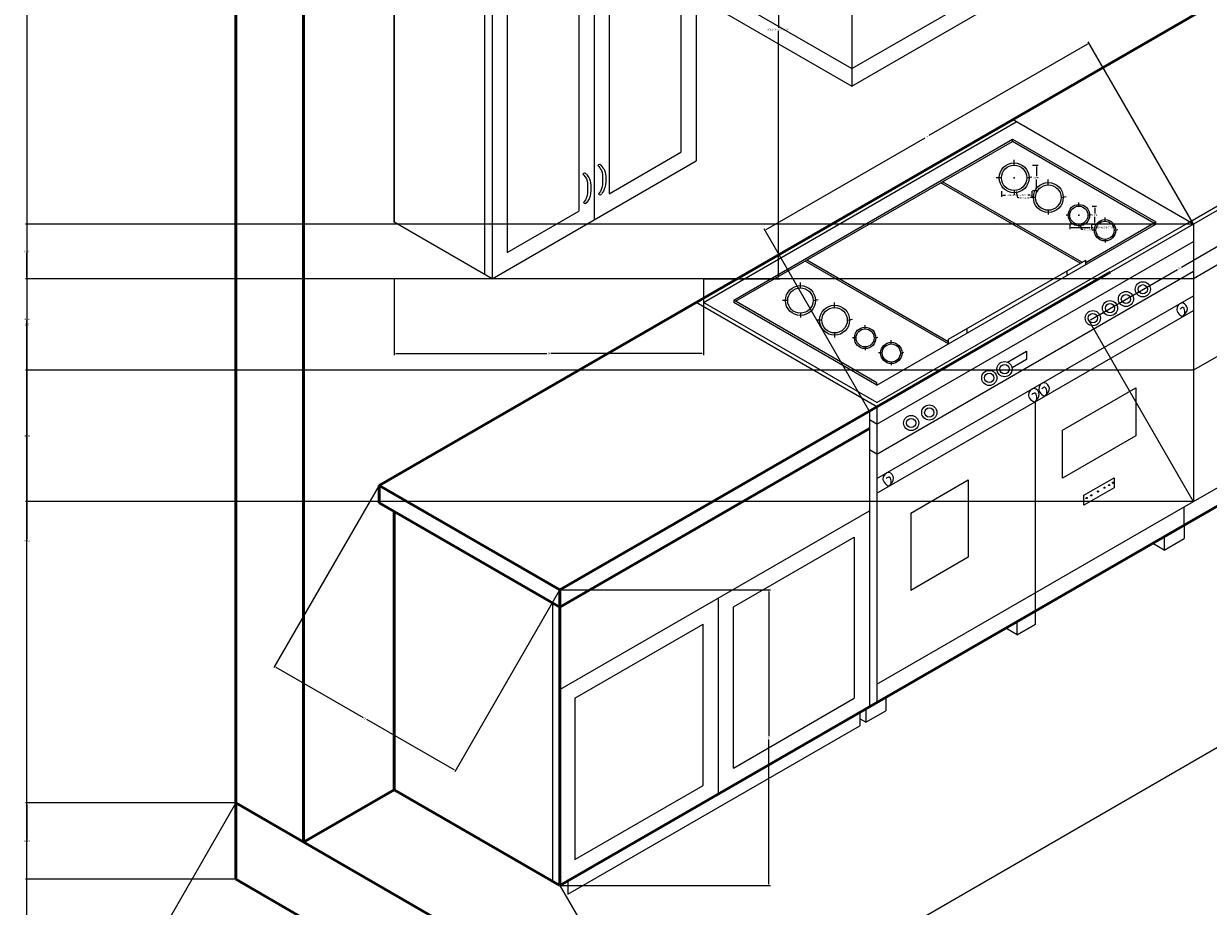
# Model space of a CAD drawing. Units: inches. Extents: x 4150 to 4636, y 2169 to 2592.
# Tile 2 of 8: x 4150 to 4286, y 2337 to 2438. Entities that reach past the tile are written whole.
import ezdxf

# ---------------------------------------------------------------- set-up
doc = ezdxf.new("R2010")
doc.units = ezdxf.units.IN
for name, color, linetype, lineweight in [('A-ANNO-DIMS', 2, 'Continuous', 18), ('A-EQPM', 6, 'Continuous', 25), ('A-FLOR-CASE', 3, 'Continuous', 25), ('A-FLOR-FIXT', 8, 'Continuous', 18), ('A-WALL', 7, 'Continuous', 50)]:
    doc.layers.add(name, color=color, linetype=linetype, lineweight=lineweight)
doc.styles.get("Standard").update_dxf_attribs({"font": 'arial.ttf'})
doc.dimstyles.get("Standard").update_dxf_attribs({"dimtxt": 0.18, "dimasz": 0.18, "dimexe": 0.18, "dimexo": 0.0625, "dimgap": 0.09, "dimtad": 0, "dimtih": 1, "dimtoh": 1, "dimdec": 4, "dimzin": 0, "dimdsep": 46, "dimtxsty": 'Standard', "dimcen": 0.09, "dimadec": 0, "dimazin": 0, "dimtfac": 1, "dimtdec": 4, "dimtofl": 0, "dimtmove": 0, "dimatfit": 3, "dimfxl": 1, "dimtolj": 1, "dimtzin": 0, "dimarcsym": 0})

# ---------------------------------------------------------------- blocks, each defined once
blk = doc.blocks.new('CUBOARD 2')
for p, q in [((4217.63, 2465.79), (4218.5, 2466.29)), ((4217.63, 2463.68), (4217.63, 2465.79)), ((4226.29, 2460.79), (4217.63, 2465.79)), ((4228.02, 2460.79), (4218.5, 2466.29)), ((4195.16, 2450.71), (4217.63, 2463.68)), ((4224.46, 2459.74), (4217.63, 2463.68)), ((4201.99, 2446.77), (4226.29, 2460.79)), ((4202.86, 2446.27), (4228.02, 2460.79)), ((4202.86, 2446.27), (4228.02, 2460.79)), ((4228.02, 2460.79), (4228.02, 2457.68)), ((4202.86, 2443.15), (4228.02, 2457.68)), ((4227.16, 2457.18), (4227.16, 2422.52)), ((4217.17, 2449.42), (4225.43, 2454.18)), ((4225.43, 2454.18), (4225.43, 2423.52)), ((4192.47, 2452.27), (4202.86, 2446.27)), ((4192.47, 2449.15), (4192.47, 2452.27)), ((4215.44, 2450.42), (4215.44, 2415.75)), ((4192.47, 2449.15), (4202.86, 2443.15)), ((4192.47, 2449.15), (4192.47, 2415.49)), ((4217.17, 2449.42), (4217.17, 2418.75)), ((4205.46, 2442.65), (4213.71, 2447.42)), ((4213.71, 2447.42), (4213.71, 2416.75)), ((4202.86, 2446.27), (4202.86, 2443.15)), ((4202.86, 2443.15), (4202.86, 2446.27)), ((4203.72, 2443.65), (4203.72, 2408.99)), ((4202.86, 2443.15), (4202.86, 2409.49)), ((4205.46, 2442.65), (4205.46, 2411.99)), ((4217.17, 2418.75), (4225.43, 2423.52)), ((4203.72, 2408.99), (4227.16, 2422.52)), ((4205.46, 2411.99), (4213.71, 2416.75)), ((4203.72, 2408.99), (4192.47, 2415.49))]:
    blk.add_line(p, q)
for centre, radius, start, end in [((4216.06, 2421.92), 0.201, 29.3135, 156.7087), ((4214.34, 2420.93), 0.201, 29.3135, 156.7087), ((4214.42, 2417.84), 0.198, 207.8897, 338.1325), ((4216.13, 2418.83), 0.198, 207.8897, 338.1325)]:
    blk.add_arc(centre, radius, start, end)
for points in [[(4215.87, 2422), (4216.03, 2421.82), (4216.41, 2421.39), (4216.43, 2420.34), (4216.42, 2419.36), (4216.06, 2418.86), (4215.96, 2418.73)], [(4216.23, 2422.02), (4216.39, 2421.84), (4216.77, 2421.41), (4216.79, 2420.36), (4216.78, 2419.38), (4216.41, 2418.88), (4216.32, 2418.75)], [(4214.16, 2421.01), (4214.31, 2420.83), (4214.69, 2420.4), (4214.71, 2419.35), (4214.71, 2418.37), (4214.34, 2417.87), (4214.24, 2417.74)], [(4214.52, 2421.03), (4214.67, 2420.85), (4215.05, 2420.42), (4215.07, 2419.37), (4215.07, 2418.38), (4214.7, 2417.89), (4214.6, 2417.76)]]:
    blk.add_open_spline(points, degree=3, knots=[0, 0, 0, 0, 0.695815, 1.679053, 3.025679, 3.502598, 3.502598, 3.502598, 3.502598])
blk = doc.blocks.new('AIR FRESH')
for p, q in [((4253.73, 2486.84), (4245.07, 2491.84)), ((4236.41, 2486.84), (4236.41, 2462.84)), ((4245.07, 2481.84), (4236.41, 2486.84)), ((4245.07, 2481.84), (4253.73, 2486.84)), ((4253.73, 2486.84), (4253.73, 2462.84)), ((4245.07, 2457.84), (4245.07, 2481.84)), ((4238.41, 2480.59), (4238.41, 2478.46)), ((4238.41, 2480.59), (4242.22, 2478.39)), ((4238.41, 2478.46), (4242.22, 2476.26)), ((4242.22, 2476.26), (4242.22, 2478.39)), ((4236.41, 2462.84), (4228.02, 2457.99)), ((4236.41, 2462.84), (4245.07, 2457.84)), ((4253.73, 2462.84), (4245.07, 2457.84)), ((4253.73, 2462.84), (4275.13, 2450.48)), ((4245.07, 2457.84), (4245.07, 2433.13)), ((4245.07, 2433.13), (4275.13, 2450.48)), ((4275.13, 2450.48), (4275.13, 2448.48)), ((4245.07, 2431.13), (4275.13, 2448.48)), ((4227.16, 2443.47), (4245.07, 2433.13)), ((4227.16, 2441.47), (4245.07, 2431.13)), ((4245.07, 2433.13), (4245.07, 2431.13))]:
    blk.add_line(p, q)
for centre in [(4239.24, 2478.91), (4240.29, 2478.31), (4241.32, 2477.71)]:
    blk.add_circle(centre, 0.313)
blk = doc.blocks.new('KNOB-A')
blk.add_line((2.93, 1.46), (3.5, 1.57))
blk.add_circle((1.46, 1.46), 1.46)
blk = doc.blocks.new('KNOB-B')
blk.add_line((2.09, 1.04), (2.5, 1.12))
blk.add_circle((1.04, 1.04), 1.04)
blk = doc.blocks.new('*D26')
at = {"layer": 'A-ANNO-DIMS', "color": 0, "lineweight": -2, "transparency": 16777216}
for p, q in [((4262.25, 2419.06), (4262.25, 2418.41)), ((4265.75, 2419.06), (4265.75, 2418.41)), ((4262.43, 2418.59), (4262.73, 2418.59)), ((4265.57, 2418.59), (4265.27, 2418.59))]:
    blk.add_line(p, q, dxfattribs=at)
at = {"layer": 'A-ANNO-DIMS', "color": 0, "transparency": 16777216}
for points in [[(4262.43, 2418.62), (4262.43, 2418.56), (4262.25, 2418.59)], [(4265.57, 2418.62), (4265.57, 2418.56), (4265.75, 2418.59)]]:
    blk.add_solid(points, dxfattribs=at)
at = {"layer": 'Defpoints', "color": 0, "transparency": 16777216}
for p in [(4262.25, 2419.12), (4265.75, 2419.12), (4265.75, 2418.59)]:
    blk.add_point(p, dxfattribs=at)
at = {"layer": 'A-ANNO-DIMS', "color": 0, "transparency": 16777216, "insert": (4264, 2418.59), "char_height": 0.18, "attachment_point": 5}
blk.add_mtext('\\A1;HOB KNOB A 4 TYP.', dxfattribs=at)
blk = doc.blocks.new('*D27')
at = {"layer": 'A-ANNO-DIMS', "color": 0, "lineweight": -2, "transparency": 16777216}
for p, q in [((4265.81, 2422.05), (4266.46, 2422.05)), ((4266.28, 2421.87), (4266.28, 2420.77)), ((4266.28, 2419.3), (4266.28, 2420.4)), ((4265.81, 2419.12), (4266.46, 2419.12))]:
    blk.add_line(p, q, dxfattribs=at)
at = {"layer": 'A-ANNO-DIMS', "color": 0, "transparency": 16777216}
for points in [[(4266.25, 2421.87), (4266.31, 2421.87), (4266.28, 2422.05)], [(4266.25, 2419.3), (4266.31, 2419.3), (4266.28, 2419.12)]]:
    blk.add_solid(points, dxfattribs=at)
at = {"layer": 'Defpoints', "color": 0, "transparency": 16777216}
for p in [(4265.75, 2422.05), (4266.28, 2422.05), (4265.75, 2419.12)]:
    blk.add_point(p, dxfattribs=at)
at = {"layer": 'A-ANNO-DIMS', "color": 0, "transparency": 16777216, "insert": (4266.28, 2420.58), "char_height": 0.18, "attachment_point": 5}
blk.add_mtext('\\A1;3 TYP.', dxfattribs=at)
blk = doc.blocks.new('*D28')
at = {"layer": 'A-ANNO-DIMS', "color": 0, "lineweight": -2, "transparency": 16777216}
for p, q in [((4270.1, 2415.18), (4270.1, 2414.69)), ((4270.28, 2414.87), (4272.42, 2414.87)), ((4272.6, 2415.18), (4272.6, 2414.69)), ((4272.6, 2414.87), (4272.78, 2414.87))]:
    blk.add_line(p, q, dxfattribs=at)
at = {"layer": 'A-ANNO-DIMS', "color": 0, "transparency": 16777216}
for points in [[(4270.28, 2414.9), (4270.28, 2414.84), (4270.1, 2414.87)], [(4272.42, 2414.9), (4272.42, 2414.84), (4272.6, 2414.87)]]:
    blk.add_solid(points, dxfattribs=at)
at = {"layer": 'Defpoints', "color": 0, "transparency": 16777216}
for p in [(4270.1, 2415.25), (4272.6, 2415.25), (4272.6, 2414.87)]:
    blk.add_point(p, dxfattribs=at)
at = {"layer": 'A-ANNO-DIMS', "color": 0, "transparency": 16777216, "insert": (4274.05, 2414.87), "char_height": 0.18, "attachment_point": 5}
blk.add_mtext('\\A1;HOB KNOB B 2 TYP.', dxfattribs=at)
blk = doc.blocks.new('*D29')
at = {"layer": 'A-ANNO-DIMS', "color": 0, "lineweight": -2, "transparency": 16777216}
for p, q in [((4272.67, 2417.33), (4273.16, 2417.33)), ((4272.98, 2417.15), (4272.98, 2416.47)), ((4272.98, 2415.43), (4272.98, 2416.11)), ((4272.67, 2415.25), (4273.16, 2415.25))]:
    blk.add_line(p, q, dxfattribs=at)
at = {"layer": 'A-ANNO-DIMS', "color": 0, "transparency": 16777216}
for points in [[(4272.95, 2417.15), (4273.01, 2417.15), (4272.98, 2417.33)], [(4272.95, 2415.43), (4273.01, 2415.43), (4272.98, 2415.25)]]:
    blk.add_solid(points, dxfattribs=at)
at = {"layer": 'Defpoints', "color": 0, "transparency": 16777216}
for p in [(4272.6, 2417.33), (4272.98, 2417.33), (4272.6, 2415.25)]:
    blk.add_point(p, dxfattribs=at)
at = {"layer": 'A-ANNO-DIMS', "color": 0, "transparency": 16777216, "insert": (4272.98, 2416.29), "char_height": 0.18, "attachment_point": 5}
blk.add_mtext('\\A1;2 TYP.', dxfattribs=at)
blk = doc.blocks.new('*D34')
at = {"layer": 'A-ANNO-DIMS', "color": 0, "lineweight": -2, "transparency": 16777216}
for p, q in [((4228.09, 2466.29), (4236.8, 2466.29)), ((4236.62, 2466.11), (4236.62, 2437.82)), ((4236.62, 2409.17), (4236.62, 2437.46)), ((4228.09, 2408.99), (4236.8, 2408.99))]:
    blk.add_line(p, q, dxfattribs=at)
at = {"layer": 'A-ANNO-DIMS', "color": 0, "transparency": 16777216}
for points in [[(4236.59, 2466.11), (4236.65, 2466.11), (4236.62, 2466.29)], [(4236.59, 2409.17), (4236.65, 2409.17), (4236.62, 2408.99)]]:
    blk.add_solid(points, dxfattribs=at)
at = {"layer": 'Defpoints', "color": 0, "transparency": 16777216}
for p in [(4228.02, 2466.29), (4236.62, 2466.29), (4228.02, 2408.99)]:
    blk.add_point(p, dxfattribs=at)
at = {"layer": 'A-ANNO-DIMS', "color": 0, "transparency": 16777216, "insert": (4236.62, 2437.64), "char_height": 0.18, "attachment_point": 5}
blk.add_mtext('\\A1;WALL CUPBOARD 2 57', dxfattribs=at)
blk = doc.blocks.new('*D35')
at = {"layer": 'A-ANNO-DIMS', "color": 0, "lineweight": -2, "transparency": 16777216}
for p, q in [((4192.47, 2408.92), (4192.47, 2400.21)), ((4228.02, 2408.92), (4228.02, 2400.21)), ((4192.65, 2400.39), (4210.03, 2400.39)), ((4227.84, 2400.39), (4210.46, 2400.39))]:
    blk.add_line(p, q, dxfattribs=at)
at = {"layer": 'A-ANNO-DIMS', "color": 0, "transparency": 16777216}
for points in [[(4192.65, 2400.42), (4192.65, 2400.36), (4192.47, 2400.39)], [(4227.84, 2400.42), (4227.84, 2400.36), (4228.02, 2400.39)]]:
    blk.add_solid(points, dxfattribs=at)
at = {"layer": 'Defpoints', "color": 0, "transparency": 16777216}
for p in [(4192.47, 2408.99), (4228.02, 2408.99), (4228.02, 2400.39)]:
    blk.add_point(p, dxfattribs=at)
at = {"layer": 'A-ANNO-DIMS', "color": 0, "transparency": 16777216, "insert": (4210.25, 2400.39), "char_height": 0.18, "attachment_point": 5}
blk.add_mtext('\\A1;36', dxfattribs=at)
blk = doc.blocks.new('*D36')
at = {"layer": 'A-ANNO-DIMS', "color": 0, "lineweight": -2, "transparency": 16777216}
for p, q in [((4174.28, 2460.03), (4174.28, 2592.15)), ((4174.46, 2591.97), (4402.51, 2591.97)), ((4631.36, 2591.97), (4403.31, 2591.97)), ((4631.54, 2412.03), (4631.54, 2592.15))]:
    blk.add_line(p, q, dxfattribs=at)
at = {"layer": 'A-ANNO-DIMS', "color": 0, "transparency": 16777216}
for points in [[(4174.46, 2592), (4174.46, 2591.94), (4174.28, 2591.97)], [(4631.36, 2592), (4631.36, 2591.94), (4631.54, 2591.97)]]:
    blk.add_solid(points, dxfattribs=at)
at = {"layer": 'Defpoints', "color": 0, "transparency": 16777216}
for p in [(4631.54, 2591.97), (4174.28, 2459.97), (4631.54, 2411.97)]:
    blk.add_point(p, dxfattribs=at)
at = {"layer": 'A-ANNO-DIMS', "color": 0, "transparency": 16777216, "insert": (4402.91, 2591.97), "char_height": 0.18, "attachment_point": 5}
blk.add_mtext('\\A1;457.3', dxfattribs=at)
blk = doc.blocks.new('*D37')
at = {"layer": 'A-ANNO-DIMS', "color": 0, "lineweight": -2, "transparency": 16777216}
for p, q in [((4361.28, 2567.97), (4150.1, 2567.97)), ((4150.28, 2567.79), (4150.28, 2379.06)), ((4150.28, 2189.96), (4150.28, 2378.69)), ((4434.34, 2189.78), (4150.1, 2189.78))]:
    blk.add_line(p, q, dxfattribs=at)
at = {"layer": 'A-ANNO-DIMS', "color": 0, "transparency": 16777216}
for points in [[(4150.25, 2567.79), (4150.31, 2567.79), (4150.28, 2567.97)], [(4150.25, 2189.96), (4150.31, 2189.96), (4150.28, 2189.78)]]:
    blk.add_solid(points, dxfattribs=at)
at = {"layer": 'Defpoints', "color": 0, "transparency": 16777216}
for p in [(4361.34, 2567.97), (4150.28, 2189.78), (4434.4, 2189.78)]:
    blk.add_point(p, dxfattribs=at)
at = {"layer": 'A-ANNO-DIMS', "color": 0, "transparency": 16777216, "insert": (4150.28, 2378.87), "char_height": 0.18, "attachment_point": 5}
blk.add_mtext('\\A1;378.2', dxfattribs=at)
blk = doc.blocks.new('*D38')
at = {"layer": 'A-ANNO-DIMS', "color": 0, "lineweight": -2, "transparency": 16777216}
for p, q in [((4174.25, 2348.68), (4162.2, 2327.79)), ((4162.45, 2327.85), (4292.04, 2253.15)), ((4422.26, 2178.08), (4292.67, 2252.79)), ((4434.37, 2198.73), (4422.33, 2177.84))]:
    blk.add_line(p, q, dxfattribs=at)
at = {"layer": 'A-ANNO-DIMS', "color": 0, "transparency": 16777216}
for points in [[(4162.46, 2327.88), (4162.43, 2327.83), (4162.29, 2327.94)], [(4422.27, 2178.11), (4422.24, 2178.05), (4422.42, 2177.99)]]:
    blk.add_solid(points, dxfattribs=at)
at = {"layer": 'Defpoints', "color": 0, "transparency": 16777216}
for p in [(4174.28, 2348.74), (4162.29, 2327.94), (4434.4, 2198.78)]:
    blk.add_point(p, dxfattribs=at)
at = {"layer": 'A-ANNO-DIMS', "color": 0, "transparency": 16777216, "insert": (4292.35, 2252.97), "char_height": 0.18, "attachment_point": 5}
blk.add_mtext('\\A1;300.25', dxfattribs=at)
blk = doc.blocks.new('*D40')
at = {"layer": 'A-ANNO-DIMS', "color": 0, "lineweight": -2, "transparency": 16777216}
for p, q in [((4174.22, 2348.74), (4150.1, 2348.74)), ((4150.28, 2348.56), (4150.28, 2344.53)), ((4150.28, 2340.15), (4150.28, 2344.17)), ((4174.22, 2339.97), (4150.1, 2339.97))]:
    blk.add_line(p, q, dxfattribs=at)
at = {"layer": 'A-ANNO-DIMS', "color": 0, "transparency": 16777216}
for points in [[(4150.25, 2348.56), (4150.31, 2348.56), (4150.28, 2348.74)], [(4150.25, 2340.15), (4150.31, 2340.15), (4150.28, 2339.97)]]:
    blk.add_solid(points, dxfattribs=at)
at = {"layer": 'Defpoints', "color": 0, "transparency": 16777216}
for p in [(4174.28, 2348.74), (4150.28, 2339.97), (4174.28, 2339.97)]:
    blk.add_point(p, dxfattribs=at)
at = {"layer": 'A-ANNO-DIMS', "color": 0, "transparency": 16777216, "insert": (4150.28, 2344.35), "char_height": 0.18, "attachment_point": 5}
blk.add_mtext('\\A1;8.771', dxfattribs=at)
blk = doc.blocks.new('*D41')
at = {"layer": 'A-ANNO-DIMS', "color": 0, "lineweight": -2, "transparency": 16777216}
for p, q in [((4174.22, 2459.97), (4150.1, 2459.97)), ((4150.28, 2459.79), (4150.28, 2404.53)), ((4150.28, 2348.92), (4150.28, 2404.17)), ((4174.22, 2348.74), (4150.1, 2348.74))]:
    blk.add_line(p, q, dxfattribs=at)
at = {"layer": 'A-ANNO-DIMS', "color": 0, "transparency": 16777216}
for points in [[(4150.25, 2459.79), (4150.31, 2459.79), (4150.28, 2459.97)], [(4150.25, 2348.92), (4150.31, 2348.92), (4150.28, 2348.74)]]:
    blk.add_solid(points, dxfattribs=at)
at = {"layer": 'Defpoints', "color": 0, "transparency": 16777216}
for p in [(4174.28, 2459.97), (4150.28, 2348.74), (4174.28, 2348.74)]:
    blk.add_point(p, dxfattribs=at)
at = {"layer": 'A-ANNO-DIMS', "color": 0, "transparency": 16777216, "insert": (4150.28, 2404.35), "char_height": 0.18, "attachment_point": 5}
blk.add_mtext('\\A1;111.23', dxfattribs=at)
blk = doc.blocks.new('*D55')
at = {"layer": 'A-ANNO-DIMS', "color": 0, "lineweight": -2, "transparency": 16777216}
for p, q in [((4380.31, 2436.61), (4392.37, 2415.73)), ((4392.12, 2415.79), (4308.21, 2367.35)), ((4223.67, 2318.54), (4307.58, 2366.99)), ((4211.55, 2339.18), (4223.61, 2318.3))]:
    blk.add_line(p, q, dxfattribs=at)
at = {"layer": 'A-ANNO-DIMS', "color": 0, "transparency": 16777216}
for points in [[(4392.11, 2415.82), (4392.14, 2415.77), (4392.28, 2415.88)], [(4223.66, 2318.57), (4223.69, 2318.52), (4223.52, 2318.45)]]:
    blk.add_solid(points, dxfattribs=at)
at = {"layer": 'Defpoints', "color": 0, "transparency": 16777216}
for p in [(4380.28, 2436.67), (4211.52, 2339.24), (4223.52, 2318.45)]:
    blk.add_point(p, dxfattribs=at)
at = {"layer": 'A-ANNO-DIMS', "color": 0, "transparency": 16777216, "insert": (4307.9, 2367.17), "char_height": 0.18, "attachment_point": 5}
blk.add_mtext('\\A1;194.86', dxfattribs=at)
blk = doc.blocks.new('*D56')
at = {"layer": 'A-ANNO-DIMS', "color": 0, "lineweight": -2, "transparency": 16777216}
for p, q in [((4190.7, 2385.18), (4178.64, 2364.3)), ((4211.49, 2373.18), (4199.43, 2352.3)), ((4178.89, 2364.36), (4188.91, 2358.58)), ((4199.36, 2352.54), (4189.35, 2358.32))]:
    blk.add_line(p, q, dxfattribs=at)
at = {"layer": 'A-ANNO-DIMS', "color": 0, "transparency": 16777216}
for points in [[(4178.91, 2364.39), (4178.88, 2364.34), (4178.73, 2364.45)], [(4199.38, 2352.57), (4199.35, 2352.52), (4199.52, 2352.45)]]:
    blk.add_solid(points, dxfattribs=at)
at = {"layer": 'Defpoints', "color": 0, "transparency": 16777216}
for p in [(4190.73, 2385.24), (4211.52, 2373.24), (4178.73, 2364.45)]:
    blk.add_point(p, dxfattribs=at)
at = {"layer": 'A-ANNO-DIMS', "color": 0, "transparency": 16777216, "insert": (4189.13, 2358.45), "char_height": 0.18, "attachment_point": 5}
blk.add_mtext('\\A1;24', dxfattribs=at)
blk = doc.blocks.new('*D57')
at = {"layer": 'A-ANNO-DIMS', "color": 0, "lineweight": -2, "transparency": 16777216}
for p, q in [((4211.58, 2373.24), (4235.7, 2373.24)), ((4235.52, 2373.06), (4235.52, 2356.42)), ((4235.52, 2339.42), (4235.52, 2356.05)), ((4211.58, 2339.24), (4235.7, 2339.24))]:
    blk.add_line(p, q, dxfattribs=at)
at = {"layer": 'A-ANNO-DIMS', "color": 0, "transparency": 16777216}
for points in [[(4235.49, 2373.06), (4235.55, 2373.06), (4235.52, 2373.24)], [(4235.49, 2339.42), (4235.55, 2339.42), (4235.52, 2339.24)]]:
    blk.add_solid(points, dxfattribs=at)
at = {"layer": 'Defpoints', "color": 0, "transparency": 16777216}
for p in [(4211.52, 2373.24), (4211.52, 2339.24), (4235.52, 2339.24)]:
    blk.add_point(p, dxfattribs=at)
at = {"layer": 'A-ANNO-DIMS', "color": 0, "transparency": 16777216, "insert": (4235.52, 2356.24), "char_height": 0.18, "attachment_point": 5}
blk.add_mtext('\\A1;34', dxfattribs=at)
blk = doc.blocks.new('*D70')
at = {"layer": 'A-ANNO-DIMS', "color": 0, "lineweight": -2, "transparency": 16777216}
for p, q in [((4272.16, 2435.96), (4253.92, 2425.43)), ((4284.28, 2415.32), (4272.23, 2436.21)), ((4235.23, 2414.64), (4253.47, 2425.17)), ((4247.04, 2393.82), (4234.99, 2414.71))]:
    blk.add_line(p, q, dxfattribs=at)
at = {"layer": 'A-ANNO-DIMS', "color": 0, "transparency": 16777216}
for points in [[(4272.14, 2435.99), (4272.17, 2435.93), (4272.32, 2436.05)], [(4235.22, 2414.67), (4235.25, 2414.61), (4235.08, 2414.55)]]:
    blk.add_solid(points, dxfattribs=at)
at = {"layer": 'Defpoints', "color": 0, "transparency": 16777216}
for p in [(4272.32, 2436.05), (4284.32, 2415.27), (4247.08, 2393.77)]:
    blk.add_point(p, dxfattribs=at)
at = {"layer": 'A-ANNO-DIMS', "color": 0, "transparency": 16777216, "insert": (4253.7, 2425.3), "char_height": 0.18, "attachment_point": 5}
blk.add_mtext('\\A1;43', dxfattribs=at)
blk = doc.blocks.new('*D71')
at = {"layer": 'A-ANNO-DIMS', "color": 0, "lineweight": -2, "transparency": 16777216}
for p, q in [((4305.07, 2395.43), (4293.01, 2416.32)), ((4292.94, 2416.07), (4282.93, 2410.29)), ((4272.47, 2404.25), (4282.49, 2410.04)), ((4284.28, 2383.43), (4272.23, 2404.32))]:
    blk.add_line(p, q, dxfattribs=at)
at = {"layer": 'A-ANNO-DIMS', "color": 0, "transparency": 16777216}
for points in [[(4292.93, 2416.1), (4292.96, 2416.05), (4293.1, 2416.16)], [(4272.46, 2404.28), (4272.49, 2404.23), (4272.32, 2404.16)]]:
    blk.add_solid(points, dxfattribs=at)
at = {"layer": 'Defpoints', "color": 0, "transparency": 16777216}
for p in [(4293.1, 2416.16), (4305.1, 2395.38), (4284.32, 2383.38)]:
    blk.add_point(p, dxfattribs=at)
at = {"layer": 'A-ANNO-DIMS', "color": 0, "transparency": 16777216, "insert": (4282.71, 2410.16), "char_height": 0.18, "attachment_point": 5}
blk.add_mtext('\\A1;24', dxfattribs=at)
blk = doc.blocks.new('*D72')
at = {"layer": 'A-ANNO-DIMS', "color": 0, "lineweight": -2, "transparency": 16777216}
for p, q in [((4284.25, 2415.27), (4150.1, 2415.27)), ((4150.28, 2415.09), (4150.28, 2412.3)), ((4150.28, 2409.16), (4150.28, 2411.94)), ((4284.25, 2408.98), (4150.1, 2408.98))]:
    blk.add_line(p, q, dxfattribs=at)
at = {"layer": 'A-ANNO-DIMS', "color": 0, "transparency": 16777216}
for points in [[(4150.25, 2415.09), (4150.31, 2415.09), (4150.28, 2415.27)], [(4150.25, 2409.16), (4150.31, 2409.16), (4150.28, 2408.98)]]:
    blk.add_solid(points, dxfattribs=at)
at = {"layer": 'Defpoints', "color": 0, "transparency": 16777216}
for p in [(4284.32, 2415.27), (4150.28, 2408.98), (4284.32, 2408.98)]:
    blk.add_point(p, dxfattribs=at)
at = {"layer": 'A-ANNO-DIMS', "color": 0, "transparency": 16777216, "insert": (4150.28, 2412.12), "char_height": 0.18, "attachment_point": 5}
blk.add_mtext('\\A1;6.285', dxfattribs=at)
blk = doc.blocks.new('*D73')
at = {"layer": 'A-ANNO-DIMS', "color": 0, "lineweight": -2, "transparency": 16777216}
for p, q in [((4284.25, 2408.98), (4150.1, 2408.98)), ((4150.28, 2408.8), (4150.28, 2403.91)), ((4150.28, 2398.66), (4150.28, 2403.55)), ((4284.25, 2398.48), (4150.1, 2398.48))]:
    blk.add_line(p, q, dxfattribs=at)
at = {"layer": 'A-ANNO-DIMS', "color": 0, "transparency": 16777216}
for points in [[(4150.25, 2408.8), (4150.31, 2408.8), (4150.28, 2408.98)], [(4150.25, 2398.66), (4150.31, 2398.66), (4150.28, 2398.48)]]:
    blk.add_solid(points, dxfattribs=at)
at = {"layer": 'Defpoints', "color": 0, "transparency": 16777216}
for p in [(4284.32, 2408.98), (4150.28, 2398.48), (4284.32, 2398.48)]:
    blk.add_point(p, dxfattribs=at)
at = {"layer": 'A-ANNO-DIMS', "color": 0, "transparency": 16777216, "insert": (4150.28, 2403.73), "char_height": 0.18, "attachment_point": 5}
blk.add_mtext('\\A1;10.5', dxfattribs=at)
blk = doc.blocks.new('*D74')
at = {"layer": 'A-ANNO-DIMS', "color": 0, "lineweight": -2, "transparency": 16777216}
for p, q in [((4284.25, 2398.48), (4150.1, 2398.48)), ((4150.28, 2398.3), (4150.28, 2391.11)), ((4150.28, 2383.56), (4150.28, 2390.75)), ((4284.25, 2383.38), (4150.1, 2383.38))]:
    blk.add_line(p, q, dxfattribs=at)
at = {"layer": 'A-ANNO-DIMS', "color": 0, "transparency": 16777216}
for points in [[(4150.25, 2398.3), (4150.31, 2398.3), (4150.28, 2398.48)], [(4150.25, 2383.56), (4150.31, 2383.56), (4150.28, 2383.38)]]:
    blk.add_solid(points, dxfattribs=at)
at = {"layer": 'Defpoints', "color": 0, "transparency": 16777216}
for p in [(4284.32, 2398.48), (4150.28, 2383.38), (4284.32, 2383.38)]:
    blk.add_point(p, dxfattribs=at)
at = {"layer": 'A-ANNO-DIMS', "color": 0, "transparency": 16777216, "insert": (4150.28, 2390.93), "char_height": 0.18, "attachment_point": 5}
blk.add_mtext('\\A1;15.102', dxfattribs=at)
blk = doc.blocks.new('*D79')
at = {"layer": 'A-ANNO-DIMS', "color": 0, "lineweight": -2, "transparency": 16777216}
for p, q in [((4263.62, 2420.58), (4263.8, 2420.58)), ((4263.71, 2420.49), (4263.71, 2420.67)), ((4264.12, 2418.28), (4264, 2418.96)), ((4264.3, 2418.28), (4264.12, 2418.28))]:
    blk.add_line(p, q, dxfattribs=at)
at = {"layer": 'A-ANNO-DIMS', "color": 0, "transparency": 16777216}
blk.add_solid([(4264.03, 2418.97), (4263.97, 2418.96), (4263.97, 2419.14)], dxfattribs=at)
at = {"layer": 'Defpoints', "color": 0, "transparency": 16777216}
for p in [(4263.46, 2422.02), (4263.97, 2419.14)]:
    blk.add_point(p, dxfattribs=at)
at = {"layer": 'A-ANNO-DIMS', "color": 0, "transparency": 16777216, "insert": (4264.98, 2418.28), "char_height": 0.18, "attachment_point": 5}
blk.add_mtext('\\A1;4X ∅2.927', dxfattribs=at)
blk = doc.blocks.new('*D80')
at = {"layer": 'A-ANNO-DIMS', "color": 0, "lineweight": -2, "transparency": 16777216}
for p, q in [((4271.06, 2416.29), (4271.24, 2416.29)), ((4271.15, 2416.2), (4271.15, 2416.38)), ((4271.44, 2414.64), (4271.36, 2415.08)), ((4271.62, 2414.64), (4271.44, 2414.64))]:
    blk.add_line(p, q, dxfattribs=at)
at = {"layer": 'A-ANNO-DIMS', "color": 0, "transparency": 16777216}
blk.add_solid([(4271.39, 2415.09), (4271.33, 2415.08), (4271.33, 2415.26)], dxfattribs=at)
at = {"layer": 'Defpoints', "color": 0, "transparency": 16777216}
for p in [(4270.97, 2417.32), (4271.33, 2415.26)]:
    blk.add_point(p, dxfattribs=at)
at = {"layer": 'A-ANNO-DIMS', "color": 0, "transparency": 16777216, "insert": (4272.23, 2414.64), "char_height": 0.18, "attachment_point": 5}
blk.add_mtext('\\A1;4X ∅2.09', dxfattribs=at)

msp = doc.modelspace()

# ---------------------------------------------------------------- linework, layer by layer
at = {"layer": 'A-EQPM'}
for p, q in [((4231.4898, 2406.5115), (4263.5306, 2425.0102)), ((4231.702, 2406.389), (4263.5306, 2424.7653)), ((4263.5306, 2424.7653), (4263.5306, 2425.0102)), ((4263.5306, 2425.0102), (4279.985, 2415.5102)), ((4279.7707, 2415.389), (4263.5306, 2424.7653)), ((4263.7138, 2422.0467), (4263.7138, 2422.6384)), ((4262.2503, 2420.5833), (4261.6504, 2420.5919)), ((4267.6405, 2419.7797), (4267.6405, 2420.3713)), ((4271.3115, 2410.7729), (4255.3033, 2420.0153)), ((4271.4908, 2410.8764), (4255.4826, 2420.1188)), ((4263.7138, 2419.1198), (4263.7138, 2418.6173)), ((4266.177, 2418.3162), (4265.5771, 2418.3248)), ((4271.1495, 2417.3349), (4271.1495, 2417.7572)), ((4267.6405, 2416.8527), (4267.6405, 2416.3502)), ((4270.1049, 2416.2902), (4269.6767, 2416.2964)), ((4247.9421, 2396.7653), (4279.985, 2415.2653)), ((4271.1495, 2415.2456), (4271.1495, 2414.887)), ((4271.937, 2410.8663), (4279.985, 2415.5128)), ((4274.1576, 2415.5982), (4274.1576, 2416.0205)), ((4279.985, 2415.2653), (4279.985, 2415.5102)), ((4273.1129, 2414.5535), (4272.6847, 2414.5597)), ((4274.1576, 2413.5089), (4274.1576, 2413.1503)), ((4247.9421, 2392.2653), (4284.3152, 2413.2653)), ((4256.1693, 2401.5153), (4239.7149, 2411.0153)), ((4256.1693, 2401.5153), (4239.7149, 2411.0153)), ((4256.1342, 2401.7425), (4239.8941, 2411.1188)), ((4256.1693, 2402.0306), (4271.937, 2411.1341)), ((4271.937, 2410.6188), (4271.937, 2411.1341)), ((4247.9421, 2388.8401), (4284.3152, 2409.8401)), ((4269.7581, 2409.8761), (4269.7581, 2409.3607)), ((4239.1566, 2407.9451), (4239.1566, 2408.5368)), ((4247.9421, 2386.0208), (4284.3152, 2407.0208)), ((4231.4898, 2406.5115), (4231.4876, 2406.2653)), ((4247.9421, 2396.7653), (4231.4876, 2406.2653)), ((4247.9421, 2397.0128), (4231.4898, 2406.5115)), ((4237.6931, 2406.4816), (4237.0931, 2406.4903)), ((4243.0833, 2405.678), (4243.0833, 2406.2697)), ((4247.9421, 2384.3451), (4284.3152, 2405.3451)), ((4239.1566, 2405.0181), (4239.1566, 2404.5157)), ((4241.6198, 2404.2145), (4241.0199, 2404.2232)), ((4243.0833, 2402.751), (4243.0833, 2402.2486)), ((4246.5923, 2403.2332), (4246.5923, 2403.6555)), ((4258.2906, 2403.2553), (4258.2906, 2402.74)), ((4245.5477, 2402.1886), (4245.1194, 2402.1948)), ((4246.5923, 2401.144), (4246.5923, 2400.7853)), ((4249.6003, 2401.4965), (4249.6003, 2401.9188)), ((4256.1693, 2401.5153), (4256.1693, 2402.0306)), ((4248.5557, 2400.4519), (4248.1275, 2400.4581)), ((4262.95, 2399.4003), (4265.1342, 2400.6614)), ((4265.1342, 2400.6614), (4265.1342, 2399.7211)), ((4249.6003, 2399.4073), (4249.6003, 2399.0486)), ((4265.1342, 2399.7211), (4263.4659, 2398.7579)), ((4247.9421, 2396.7653), (4247.9421, 2397.0128)), ((4269.2822, 2391.5836), (4277.6908, 2396.4383)), ((4277.6908, 2396.4383), (4277.6908, 2390.9349)), ((4266.1286, 2394.8451), (4266.1286, 2370.7653)), ((4247.0761, 2393.7653), (4247.0761, 2359.7653)), ((4247.9421, 2392.2653), (4247.0761, 2392.7653)), ((4269.2822, 2386.0802), (4269.2822, 2391.5836)), ((4277.6908, 2390.9349), (4269.2822, 2386.0802)), ((4247.9421, 2388.8401), (4247.0761, 2389.3401)), ((4251.8296, 2382.0485), (4258.4403, 2385.8651)), ((4258.4403, 2385.8651), (4258.4403, 2376.9848)), ((4271.7331, 2384.1067), (4275.2145, 2386.1168)), ((4275.2145, 2384.9596), (4271.7331, 2382.9496)), ((4275.2145, 2386.1168), (4275.2145, 2384.9596)), ((4271.7331, 2382.9496), (4271.7331, 2384.1067)), ((4283.2299, 2380.6387), (4283.2299, 2382.7519)), ((4251.8296, 2382.0485), (4251.8296, 2373.1682)), ((4283.2299, 2380.6387), (4283.2299, 2379.1275)), ((4231.4626, 2371.2854), (4245.344, 2379.2998)), ((4245.344, 2379.2998), (4245.344, 2360.7653)), ((4280.9385, 2377.8045), (4279.6297, 2378.5601)), ((4280.939, 2379.3161), (4280.9385, 2377.8045)), ((4280.9385, 2377.8045), (4283.2299, 2379.1275)), ((4258.4403, 2376.9848), (4251.8296, 2373.1682)), ((4231.4626, 2352.7508), (4231.4626, 2371.2854)), ((4266.1286, 2370.7653), (4266.1286, 2369.254)), ((4264.0742, 2368.0679), (4262.7654, 2368.8235)), ((4264.0742, 2368.0679), (4264.0742, 2369.5791)), ((4266.1286, 2369.254), (4264.0742, 2368.0679)), ((4264.0742, 2368.0679), (4266.1286, 2369.254)), ((4231.4626, 2352.7508), (4245.344, 2360.7653))]:
    msp.add_line(p, q, dxfattribs=at)
for centre, radius in [((4263.7138, 2420.5833), 1.7199), ((4267.6405, 2418.3162), 1.7199), ((4271.1495, 2416.2902), 1.2276), ((4274.1576, 2414.5535), 1.2276), ((4239.1566, 2406.4816), 1.7199), ((4278.4975, 2407.7718), 0.8698), ((4278.4975, 2407.7718), 0.5331), ((4276.5614, 2406.6539), 0.8698), ((4276.5614, 2406.6539), 0.5331), ((4243.0833, 2404.2145), 1.7199), ((4272.757, 2404.4575), 0.8698), ((4274.7271, 2405.595), 0.8698), ((4274.7271, 2405.595), 0.5331), ((4272.757, 2404.4575), 0.5331), ((4246.5923, 2402.1886), 1.2276), ((4249.6003, 2400.4519), 1.2276), ((4260.854, 2397.5853), 0.8698), ((4262.6107, 2398.5995), 0.8698), ((4262.6107, 2398.5995), 0.5331), ((4260.854, 2397.5853), 0.5331), ((4253.9624, 2393.6064), 0.8698), ((4251.8771, 2392.4025), 0.8698), ((4253.9624, 2393.6064), 0.5331), ((4251.8771, 2392.4025), 0.5331), ((4274.0995, 2384.9736), 0.0709), ((4274.6255, 2385.2772), 0.0709), ((4275.0768, 2385.5378), 0.0709), ((4272.0371, 2383.7828), 0.0709), ((4272.5702, 2384.0906), 0.0709), ((4273.3449, 2384.5379), 0.0709)]:
    msp.add_circle(centre, radius, dxfattribs=at)
for points in [[(4283.0395, 2404.6086), (4283.3465, 2404.8935), (4283.884, 2405.3925), (4283.0866, 2406.5693), (4281.9101, 2405.4192), (4283.5292, 2404.0968), (4283.3215, 2405.9384), (4282.8922, 2405.6012), (4282.7698, 2405.5051)], [(4267.179, 2395.4515), (4267.486, 2395.7365), (4268.0235, 2396.2355), (4267.2261, 2397.4122), (4266.0496, 2396.2621), (4267.6688, 2394.9398), (4267.461, 2396.7813), (4267.0317, 2396.4442), (4266.9093, 2396.3481)], [(4266.0079, 2394.7753), (4266.3148, 2395.0603), (4266.8523, 2395.5593), (4266.055, 2396.7361), (4264.8785, 2395.586), (4266.4976, 2394.2636), (4266.2898, 2396.1052), (4265.8605, 2395.768), (4265.7381, 2395.6719)], [(4249.2809, 2385.118), (4249.5879, 2385.403), (4250.1254, 2385.902), (4249.328, 2387.0788), (4248.1515, 2385.9287), (4249.7707, 2384.6063), (4249.5629, 2386.4479), (4249.1336, 2386.1107), (4249.0112, 2386.0146)]]:
    msp.add_open_spline(points, degree=3, knots=[0, 0, 0, 0, 1.10388683, 1.93279179, 2.9808053, 4.07156191, 5.03758171, 5.42287318, 5.42287318, 5.42287318, 5.42287318], dxfattribs=at)
at = {"layer": 'A-FLOR-CASE'}
for p, q in [((4192.4665, 2415.4873), (4192.4665, 2452.2661)), ((4305.0998, 2420.9804), (4284.3152, 2408.9803)), ((4305.0998, 2410.4804), (4284.3152, 2398.4803)), ((4211.5191, 2361.771), (4247.0761, 2382.2998)), ((4210.653, 2371.7364), (4210.653, 2339.7364)), ((4229.7306, 2349.7508), (4229.7306, 2372.2854)), ((4213.2511, 2360.771), (4227.9985, 2369.2854)), ((4227.9985, 2350.7508), (4227.9985, 2369.2854)), ((4213.2511, 2360.771), (4213.2511, 2342.2364)), ((4248.9541, 2360.8495), (4248.9541, 2359.3383)), ((4245.9703, 2359.1268), (4245.9703, 2357.6156)), ((4246.6633, 2359.5269), (4246.6627, 2358.0154)), ((4246.6627, 2358.0154), (4248.9541, 2359.3383)), ((4212.4464, 2338.2606), (4245.9703, 2357.6156)), ((4246.6627, 2358.0154), (4245.9703, 2358.4152)), ((4213.2511, 2342.2364), (4227.9985, 2350.7508)), ((4212.4464, 2339.7718), (4212.4464, 2338.2606))]:
    msp.add_line(p, q, dxfattribs=at)
at = {"layer": 'A-FLOR-FIXT'}
for p, q in [((4283.8821, 2415.5153), (4381.6931, 2471.9864)), ((4247.9421, 2394.2653), (4382.1261, 2471.7364)), ((4227.1575, 2406.2653), (4263.5306, 2427.2653)), ((4228.0235, 2406.2653), (4263.9636, 2427.0153)), ((4247.9421, 2394.2653), (4305.0998, 2427.2653)), ((4284.3152, 2415.2653), (4263.5306, 2427.2653)), ((4247.9421, 2394.7653), (4283.8821, 2415.5153)), ((4284.3152, 2415.2653), (4284.3152, 2383.3785)), ((4247.9421, 2394.2653), (4227.1575, 2406.2653)), ((4247.9421, 2394.7653), (4228.0235, 2406.2653)), ((4284.3152, 2383.3785), (4305.0998, 2395.3785)), ((4247.9421, 2394.2653), (4247.9421, 2360.2653)), ((4247.9421, 2362.3785), (4284.3152, 2383.3785))]:
    msp.add_line(p, q, dxfattribs=at)
at = {"layer": 'A-WALL'}
for p, q in [((4174.28, 2339.9652), (4174.28, 2459.9652)), ((4182.0742, 2344.2364), (4182.0742, 2455.4652)), ((4190.7345, 2385.2364), (4289.9267, 2442.5051)), ((4211.5191, 2373.2364), (4274.7389, 2409.7364)), ((4211.5191, 2371.2364), (4247.0761, 2391.7653)), ((4284.3152, 2381.2653), (4303.7162, 2392.4665)), ((4190.7345, 2385.2364), (4192.4665, 2384.2364)), ((4190.7345, 2383.2364), (4190.7345, 2385.2364)), ((4192.4665, 2384.2364), (4211.5191, 2373.2364)), ((4190.7345, 2383.2364), (4211.5191, 2371.2364)), ((4192.4665, 2350.2364), (4192.4665, 2382.2364)), ((4211.5191, 2339.2364), (4284.3152, 2381.2653)), ((4211.5191, 2373.2364), (4211.5191, 2371.2364)), ((4211.5191, 2371.2364), (4211.5191, 2339.2364)), ((4182.0742, 2344.2364), (4192.4665, 2350.2364)), ((4211.5191, 2339.2364), (4192.4665, 2350.2364)), ((4174.28, 2348.7364), (4434.204, 2198.6692)), ((4174.28, 2339.9652), (4182.0742, 2335.4652))]:
    msp.add_line(p, q, dxfattribs=at)

# ---------------------------------------------------------------- block references
at = {"layer": 'A-EQPM'}
for name, p in [('AIR FRESH', (0, 0)), ('KNOB-A', (4262.25, 2419.12)), ('KNOB-A', (4266.1767, 2416.8529)), ('KNOB-B', (4270.105, 2415.246)), ('KNOB-B', (4273.113, 2413.5093)), ('KNOB-A', (4237.6928, 2405.0183)), ('KNOB-A', (4241.6195, 2402.7512)), ('KNOB-B', (4245.5478, 2401.1443)), ('KNOB-B', (4248.5558, 2399.4076))]:
    msp.add_blockref(name, p, dxfattribs=at)
at = {"layer": 'A-FLOR-CASE'}
msp.add_blockref('CUBOARD 2', (0, 0), dxfattribs=at)

# ---------------------------------------------------------------- dimensions: what is measured, and where the dimension line sits
at = {"layer": 'A-ANNO-DIMS'}
for base, p1, p2, override, picture, middle in [((4631.5414, 2591.9652), (4174.28, 2459.9652), (4631.5414, 2411.9652), {"dimdec": 1, "dimlfac": 1, "dimrnd": 0, "dimzin": 0, "dimdsep": 46, "dimlunit": 2}, '*D36', (4402.9107, 2591.9652)), ((4228.0235, 2400.3912), (4192.4665, 2408.9873), (4228.0235, 2408.9873), {"dimdec": 0, "dimlfac": 1, "dimrnd": 0, "dimzin": 0, "dimdsep": 46, "dimlunit": 2}, '*D35', (4210.245, 2400.3912))]:
    dim = msp.add_linear_dim(base=base, p1=p1, p2=p2, dimstyle='Standard', override=override, dxfattribs=at)
    dim.commit()
    dim.dimension.update_dxf_attribs({"geometry": picture, "text_midpoint": middle})
for base, p1, p2, angle, override, picture, middle in [((4150.28, 2189.7836), (4361.3415, 2567.9652), (4434.4021, 2189.7836), 90, {"dimdec": 1, "dimlfac": 1, "dimrnd": 0, "dimzin": 0, "dimdsep": 46, "dimlunit": 2}, '*D37', (4150.28, 2378.8744)), ((4150.28, 2348.7364), (4174.28, 2459.9652), (4174.28, 2348.7364), 90, {"dimdec": 2, "dimlfac": 1, "dimrnd": 0, "dimzin": 0, "dimdsep": 46, "dimlunit": 2}, '*D41', (4150.28, 2404.3508)), ((4223.5191, 2318.4518), (4380.2767, 2436.6687), (4211.5191, 2339.2364), 210, {"dimdec": 2, "dimlfac": 1, "dimrnd": 0, "dimzin": 0, "dimdsep": 46, "dimlunit": 2}, '*D55', (4307.8979, 2367.1679)), ((4272.3152, 2436.0499), (4247.0761, 2393.7653), (4284.3152, 2415.2653), 30, {"dimdec": 0, "dimlfac": 1, "dimrnd": 0, "dimzin": 0, "dimdsep": 46, "dimlunit": 2}, '*D70', (4253.6956, 2425.2999)), ((4293.0998, 2416.1631), (4284.3152, 2383.3785), (4305.0998, 2395.3785), 30, {"dimdec": 0, "dimlfac": 1, "dimrnd": 0, "dimzin": 0, "dimdsep": 46, "dimlunit": 2}, '*D71', (4282.7075, 2410.1631)), ((4150.28, 2408.9803), (4284.3152, 2415.2653), (4284.3152, 2408.9803), 90, {"dimdec": 3, "dimlfac": 1, "dimrnd": 0, "dimzin": 0, "dimdsep": 46, "dimlunit": 2}, '*D72', (4150.28, 2412.1228)), ((4150.28, 2398.4803), (4284.3152, 2408.9803), (4284.3152, 2398.4803), 90, {"dimdec": 1, "dimlfac": 1, "dimrnd": 0, "dimzin": 0, "dimdsep": 46, "dimlunit": 2}, '*D73', (4150.28, 2403.7303)), ((4150.28, 2383.3785), (4284.3152, 2398.4803), (4284.3152, 2383.3785), 90, {"dimdec": 3, "dimlfac": 1, "dimrnd": 0, "dimzin": 0, "dimdsep": 46, "dimlunit": 2}, '*D74', (4150.28, 2390.9294)), ((4178.7345, 2364.4518), (4211.5191, 2373.2364), (4190.7345, 2385.2364), 150, {"dimdec": 0, "dimlfac": 1, "dimrnd": 0, "dimzin": 0, "dimdsep": 46, "dimlunit": 2}, '*D56', (4189.1268, 2358.4518)), ((4235.5191, 2339.2364), (4211.5191, 2373.2364), (4211.5191, 2339.2364), 270, {"dimdec": 0, "dimlfac": 1, "dimrnd": 0, "dimzin": 0, "dimdsep": 46, "dimlunit": 2}, '*D57', (4235.5191, 2356.2364)), ((4150.28, 2339.9652), (4174.28, 2348.7364), (4174.28, 2339.9652), 90, {"dimdec": 3, "dimlfac": 1, "dimrnd": 0, "dimzin": 0, "dimdsep": 46, "dimlunit": 2}, '*D40', (4150.28, 2344.3508)), ((4162.2937, 2327.9439), (4434.4021, 2198.7836), (4174.28, 2348.7364), 150.037803, {"dimdec": 2, "dimlfac": 1, "dimrnd": 0, "dimzin": 0, "dimdsep": 46, "dimlunit": 2}, '*D38', (4292.3547, 2252.9675))]:
    dim = msp.add_linear_dim(base=base, p1=p1, p2=p2, angle=angle, dimstyle='Standard', override=override, dxfattribs=at)
    dim.commit()
    dim.dimension.update_dxf_attribs({"geometry": picture, "text_midpoint": middle})
for base, p1, p2, text, picture, middle in [((4236.6197, 2466.2949), (4228.0235, 2408.9873), (4228.0235, 2466.2949), 'WALL CUPBOARD 2 <>', '*D34', (4236.6197, 2437.6411)), ((4266.2762, 2422.0467), (4265.751, 2419.1198), (4265.751, 2422.0467), '<> TYP.', '*D27', (4266.2762, 2420.5833)), ((4272.9785, 2417.3349), (4272.6036, 2415.2456), (4272.6036, 2417.3349), '<> TYP.', '*D29', (4272.9785, 2416.2902))]:
    dim = msp.add_linear_dim(base=base, p1=p1, p2=p2, angle=90, text=text, dimstyle='Standard', override={"dimdec": 0, "dimlfac": 1, "dimrnd": 0, "dimzin": 0, "dimdsep": 46, "dimlunit": 2}, dxfattribs=at)
    dim.commit()
    dim.dimension.update_dxf_attribs({"geometry": picture, "text_midpoint": middle})
for p1, p2, override, picture, middle in [((4263.4614, 2422.0248), (4263.9662, 2419.1417), {"dimdec": 3, "dimlfac": 1, "dimrnd": 0, "dimzin": 0, "dimdsep": 46, "dimlunit": 2}, '*D79', (4264.9815, 2418.2768)), ((4270.9709, 2417.3195), (4271.3281, 2415.261), {"dimdec": 2, "dimlfac": 1, "dimrnd": 0, "dimzin": 0, "dimdsep": 46, "dimlunit": 2}, '*D80', (4272.2293, 2414.6435))]:
    dim = msp.add_diameter_dim_2p(p1=p1, p2=p2, text='4X <>', dimstyle='Standard', override=override, dxfattribs=at)
    dim.commit()
    dim.dimension.update_dxf_attribs({"geometry": picture, "text_midpoint": middle, "dimtype": 163})
for base, p1, p2, text, picture, middle in [((4265.751, 2418.5947), (4262.2503, 2419.1198), (4265.751, 2419.1198), 'HOB KNOB A <> TYP.', '*D26', (4264.0007, 2418.5947)), ((4272.6036, 2414.8708), (4270.1049, 2415.2456), (4272.6036, 2415.2456), 'HOB KNOB B <> TYP.', '*D28', (4274.0544, 2414.8708))]:
    dim = msp.add_linear_dim(base=base, p1=p1, p2=p2, text=text, dimstyle='Standard', override={"dimdec": 0, "dimlfac": 1, "dimrnd": 0, "dimzin": 0, "dimdsep": 46, "dimlunit": 2}, dxfattribs=at)
    dim.commit()
    dim.dimension.update_dxf_attribs({"geometry": picture, "text_midpoint": middle})

doc.saveas('drawing.dxf')
